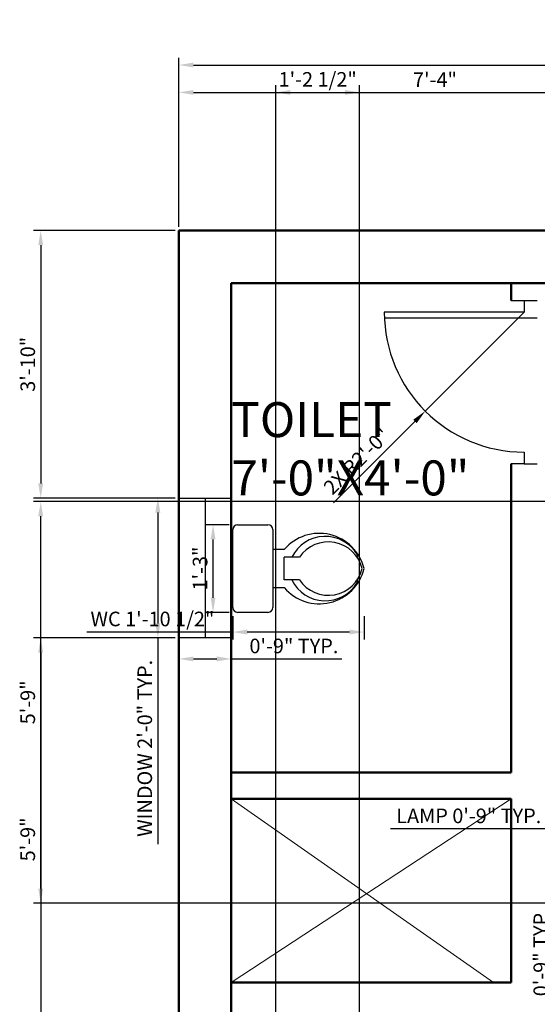
# Model space of a CAD drawing. Units: inches. Extents: x 3242 to 3618, y 1365 to 1814.
# Tile 4 of 6: x 3244 to 3333, y 1626 to 1795. Entities that reach past the tile are written whole.
import ezdxf

# ---------------------------------------------------------------- set-up
doc = ezdxf.new("R2010")
doc.units = ezdxf.units.IN
for name, color, linetype, lineweight in [('A-ANNO-DIMS', 2, 'Continuous', 18), ('A-AREA-IDEN', 7, 'Continuous', 25), ('A-DOOR', 4, 'Continuous', 25), ('A-FLOR-FIXT', 8, 'Continuous', 25), ('A-FLOR-OPEN', 1, 'Continuous', 13), ('A-GLAZ', 5, 'Continuous', 25), ('A-WALL', 7, 'Continuous', 50)]:
    doc.layers.add(name, color=color, linetype=linetype, lineweight=lineweight)
doc.styles.get("Standard").update_dxf_attribs({"font": 'arial.ttf'})
doc.dimstyles.new('ISO-25', dxfattribs={"dimtxt": 2.5, "dimasz": 2.5, "dimexe": 1.25, "dimexo": 0.625, "dimtad": 1, "dimdec": 0, "dimlunit": 3, "dimtxsty": 'Standard', "dimcen": 2.5, "dimadec": 0, "dimazin": 0, "dimtfac": 1, "dimtdec": 0, "dimtmove": 0, "dimatfit": 3, "dimfxl": 1, "dimarcsym": 0})

# ---------------------------------------------------------------- blocks, each defined once
blk = doc.blocks.new('A$C02F3725D')
for p, q in [((0.025, 0.69), (0.435, 0.69)), ((0, 0.505), (0, 0.665)), ((0.46, 0.665), (0.46, 0.505)), ((0.435, 0.48), (0.025, 0.48)), ((0.13, 0.48), (0.13, 0.42)), ((0.33, 0.42), (0.33, 0.48)), ((0.17, 0.34), (0.17, 0.42)), ((0.17, 0.42), (0.29, 0.42)), ((0.29, 0.34), (0.29, 0.42)), ((0.1578, 0.035), (0.1724, 0.035)), ((0.2876, 0.035), (0.3022, 0.035))]:
    blk.add_line(p, q)
for centre, radius, start, end in [((0.025, 0.665), 0.025, 90, 180), ((0.435, 0.665), 0.025, 0, 90), ((0.025, 0.505), 0.025, 180, 270), ((0.435, 0.505), 0.025, 270, 0), ((0.2874, 0.2356), 0.2425, 130.4885, 256.2965), ((0.1726, 0.2356), 0.2425, 283.7035, 49.5115), ((0.2568, 0.2042), 0.196, 116.2742, 239.6668), ((0.2032, 0.2042), 0.196, 300.3332, 63.7258), ((0.2732, 0.1883), 0.1834, 124.2157, 256.394), ((0.1868, 0.1883), 0.1834, 283.606, 55.7843)]:
    blk.add_arc(centre, radius, start, end)
blk = doc.blocks.new('*D3')
at = {"layer": 'A-ANNO-DIMS', "color": 0, "lineweight": -2, "transparency": 16777216}
for p, q in [((3271.48, 1759.28), (3271.48, 1788.3)), ((3592.48, 1759.28), (3592.48, 1788.3)), ((3273.98, 1787.05), (3589.98, 1787.05))]:
    blk.add_line(p, q, dxfattribs=at)
at = {"layer": 'A-ANNO-DIMS', "color": 0, "transparency": 16777216}
for points in [[(3273.98, 1787.47), (3273.98, 1786.64), (3271.48, 1787.05)], [(3589.98, 1787.47), (3589.98, 1786.64), (3592.48, 1787.05)]]:
    blk.add_solid(points, dxfattribs=at)
at = {"layer": 'Defpoints', "color": 0, "transparency": 16777216}
for p in [(3592.48, 1787.05), (3271.48, 1758.66), (3592.48, 1758.66)]:
    blk.add_point(p, dxfattribs=at)
at = {"layer": 'A-ANNO-DIMS', "color": 0, "transparency": 16777216, "insert": (3431.98, 1790.74), "char_height": 6, "attachment_point": 5}
blk.add_mtext('26\'-9"', dxfattribs=at)
blk = doc.blocks.new('DOOR-SWING-24IN')
for p, q in [((21.75, 28), (26.25, 28)), ((24, 28), (24, 26)), ((24, 26), (0, 26)), ((26.25, 25), (0, 25)), ((24, 2), (24, 0)), ((24, 0), (21.75, 0)), ((24, 0), (26.25, 0))]:
    blk.add_line(p, q)
blk.add_arc((24, 26), 24, 180, 270)
blk = doc.blocks.new('WINDOW-24IN')
for p, q in [((0, 9), (24, 9)), ((0, 0), (0, 9)), ((24, 9), (24, 0)), ((0, 4.5), (24, 4.5)), ((24, 0), (0, 0))]:
    blk.add_line(p, q)
blk = doc.blocks.new('*D15')
at = {"layer": 'A-ANNO-DIMS', "color": 0, "lineweight": -2, "transparency": 16777216}
for p, q in [((3270.86, 1712.77), (3266.63, 1712.77)), ((3267.88, 1710.27), (3267.88, 1691.27)), ((3270.86, 1688.77), (3266.63, 1688.77)), ((3267.88, 1688.77), (3267.88, 1653.38))]:
    blk.add_line(p, q, dxfattribs=at)
at = {"layer": 'A-ANNO-DIMS', "color": 0, "transparency": 16777216}
for points in [[(3267.46, 1710.27), (3268.3, 1710.27), (3267.88, 1712.77)], [(3267.46, 1691.27), (3268.3, 1691.27), (3267.88, 1688.77)]]:
    blk.add_solid(points, dxfattribs=at)
at = {"layer": 'Defpoints', "color": 0, "transparency": 16777216}
for p in [(3271.48, 1712.77), (3267.88, 1688.77), (3271.48, 1688.77)]:
    blk.add_point(p, dxfattribs=at)
at = {"layer": 'A-ANNO-DIMS', "color": 0, "transparency": 16777216, "insert": (3265.96, 1669.83), "char_height": 2.5, "attachment_point": 5, "rotation": 90}
blk.add_mtext('WINDOW 2\'-0" TYP.', dxfattribs=at)
blk = doc.blocks.new('*D16')
at = {"layer": 'A-ANNO-DIMS', "color": 0, "lineweight": -2, "transparency": 16777216}
for p, q in [((3271.48, 1688.14), (3271.48, 1683.92)), ((3280.48, 1688.14), (3280.48, 1683.92)), ((3273.98, 1685.17), (3277.98, 1685.17)), ((3280.48, 1685.17), (3299.47, 1685.17))]:
    blk.add_line(p, q, dxfattribs=at)
at = {"layer": 'A-ANNO-DIMS', "color": 0, "transparency": 16777216}
for points in [[(3273.98, 1685.59), (3273.98, 1684.75), (3271.48, 1685.17)], [(3277.98, 1685.59), (3277.98, 1684.75), (3280.48, 1685.17)]]:
    blk.add_solid(points, dxfattribs=at)
at = {"layer": 'Defpoints', "color": 0, "transparency": 16777216}
for p in [(3271.48, 1688.77), (3280.48, 1688.77), (3280.48, 1685.17)]:
    blk.add_point(p, dxfattribs=at)
at = {"layer": 'A-ANNO-DIMS', "color": 0, "transparency": 16777216, "insert": (3291.22, 1687.07), "char_height": 2.5, "attachment_point": 5}
blk.add_mtext('0\'-9" TYP.', dxfattribs=at)
blk = doc.blocks.new('*D21')
at = {"layer": 'A-ANNO-DIMS', "color": 0, "lineweight": -2, "transparency": 16777216}
for p, q in [((3280.73, 1692.53), (3280.73, 1688.53)), ((3303.26, 1692.53), (3303.26, 1688.53)), ((3280.73, 1689.78), (3255.68, 1689.78)), ((3300.76, 1689.78), (3283.23, 1689.78))]:
    blk.add_line(p, q, dxfattribs=at)
at = {"layer": 'A-ANNO-DIMS', "color": 0, "transparency": 16777216}
for points in [[(3283.23, 1690.2), (3283.23, 1689.36), (3280.73, 1689.78)], [(3300.76, 1690.2), (3300.76, 1689.36), (3303.26, 1689.78)]]:
    blk.add_solid(points, dxfattribs=at)
at = {"layer": 'Defpoints', "color": 0, "transparency": 16777216}
for p in [(3280.73, 1693.16), (3303.26, 1693.16), (3280.73, 1689.78)]:
    blk.add_point(p, dxfattribs=at)
at = {"layer": 'A-ANNO-DIMS', "color": 0, "transparency": 16777216, "insert": (3266.95, 1691.7), "char_height": 2.5, "attachment_point": 5}
blk.add_mtext('WC 1\'-10 1/2"', dxfattribs=at)
blk = doc.blocks.new('*D22')
at = {"layer": 'A-ANNO-DIMS', "color": 0, "lineweight": -2, "transparency": 16777216}
for p, q in [((3280.11, 1708.17), (3276.1, 1708.17)), ((3277.35, 1695.66), (3277.35, 1705.67)), ((3280.11, 1693.16), (3276.1, 1693.16))]:
    blk.add_line(p, q, dxfattribs=at)
at = {"layer": 'A-ANNO-DIMS', "color": 0, "transparency": 16777216}
for points in [[(3276.94, 1705.67), (3277.77, 1705.67), (3277.35, 1708.17)], [(3276.94, 1695.66), (3277.77, 1695.66), (3277.35, 1693.16)]]:
    blk.add_solid(points, dxfattribs=at)
at = {"layer": 'Defpoints', "color": 0, "transparency": 16777216}
for p in [(3277.35, 1708.17), (3280.73, 1708.17), (3280.73, 1693.16)]:
    blk.add_point(p, dxfattribs=at)
at = {"layer": 'A-ANNO-DIMS', "color": 0, "transparency": 16777216, "insert": (3275.45, 1700.67), "char_height": 2.5, "attachment_point": 5, "rotation": 90}
blk.add_mtext('1\'-3"', dxfattribs=at)
blk = doc.blocks.new('*D29')
at = {"layer": 'A-ANNO-DIMS', "color": 0, "lineweight": -2, "transparency": 16777216}
for p, q in [((3337.15, 1655.29), (3337.15, 1657.27)), ((3346.15, 1655.29), (3346.15, 1657.27)), ((3337.15, 1656.02), (3307.79, 1656.02)), ((3343.65, 1656.02), (3339.65, 1656.02))]:
    blk.add_line(p, q, dxfattribs=at)
at = {"layer": 'A-ANNO-DIMS', "color": 0, "transparency": 16777216}
for points in [[(3339.65, 1656.43), (3339.65, 1655.6), (3337.15, 1656.02)], [(3343.65, 1656.43), (3343.65, 1655.6), (3346.15, 1656.02)]]:
    blk.add_solid(points, dxfattribs=at)
at = {"layer": 'Defpoints', "color": 0, "transparency": 16777216}
for p in [(3337.15, 1656.02), (3337.15, 1654.67), (3346.15, 1654.67)]:
    blk.add_point(p, dxfattribs=at)
at = {"layer": 'A-ANNO-DIMS', "color": 0, "transparency": 16777216, "insert": (3321.22, 1657.92), "char_height": 2.5, "attachment_point": 5}
blk.add_mtext('LAMP 0\'-9" TYP.', dxfattribs=at)
blk = doc.blocks.new('*D30')
at = {"layer": 'A-ANNO-DIMS', "color": 0, "lineweight": -2, "transparency": 16777216}
for p, q in [((3336.53, 1654.67), (3334.55, 1654.67)), ((3335.8, 1652.17), (3335.8, 1648.17)), ((3336.53, 1645.67), (3334.55, 1645.67)), ((3335.8, 1645.67), (3335.8, 1626.68))]:
    blk.add_line(p, q, dxfattribs=at)
at = {"layer": 'A-ANNO-DIMS', "color": 0, "transparency": 16777216}
for points in [[(3335.39, 1652.17), (3336.22, 1652.17), (3335.8, 1654.67)], [(3335.39, 1648.17), (3336.22, 1648.17), (3335.8, 1645.67)]]:
    blk.add_solid(points, dxfattribs=at)
at = {"layer": 'Defpoints', "color": 0, "transparency": 16777216}
for p in [(3337.15, 1654.67), (3335.8, 1645.67), (3337.15, 1645.67)]:
    blk.add_point(p, dxfattribs=at)
at = {"layer": 'A-ANNO-DIMS', "color": 0, "transparency": 16777216, "insert": (3333.9, 1634.92), "char_height": 2.5, "attachment_point": 5, "rotation": 90}
blk.add_mtext('0\'-9" TYP.', dxfattribs=at)
blk = doc.blocks.new('*D33')
at = {"layer": 'A-ANNO-DIMS', "color": 0, "lineweight": -2, "transparency": 16777216}
for p, q in [((3271.48, 1759.28), (3271.48, 1783.61)), ((3273.98, 1782.36), (3356.86, 1782.36)), ((3359.36, 1759.28), (3359.36, 1783.61))]:
    blk.add_line(p, q, dxfattribs=at)
at = {"layer": 'A-ANNO-DIMS', "color": 0, "transparency": 16777216}
for points in [[(3273.98, 1782.77), (3273.98, 1781.94), (3271.48, 1782.36)], [(3356.86, 1782.77), (3356.86, 1781.94), (3359.36, 1782.36)]]:
    blk.add_solid(points, dxfattribs=at)
at = {"layer": 'Defpoints', "color": 0, "transparency": 16777216}
for p in [(3359.36, 1782.36), (3271.48, 1758.66), (3359.36, 1758.66)]:
    blk.add_point(p, dxfattribs=at)
at = {"layer": 'A-ANNO-DIMS', "color": 0, "transparency": 16777216, "insert": (3315.42, 1784.23), "char_height": 2.5, "attachment_point": 5}
blk.add_mtext('7\'-4"', dxfattribs=at)
blk = doc.blocks.new('*D37')
at = {"layer": 'A-ANNO-DIMS', "color": 0, "lineweight": -2, "transparency": 16777216}
for p, q in [((3270.86, 1758.66), (3246.53, 1758.66)), ((3247.78, 1756.16), (3247.78, 1715.27)), ((3270.86, 1712.77), (3246.53, 1712.77))]:
    blk.add_line(p, q, dxfattribs=at)
at = {"layer": 'A-ANNO-DIMS', "color": 0, "transparency": 16777216}
for points in [[(3247.36, 1756.16), (3248.2, 1756.16), (3247.78, 1758.66)], [(3247.36, 1715.27), (3248.2, 1715.27), (3247.78, 1712.77)]]:
    blk.add_solid(points, dxfattribs=at)
at = {"layer": 'Defpoints', "color": 0, "transparency": 16777216}
for p in [(3271.48, 1758.66), (3247.78, 1712.77), (3271.48, 1712.77)]:
    blk.add_point(p, dxfattribs=at)
at = {"layer": 'A-ANNO-DIMS', "color": 0, "transparency": 16777216, "insert": (3245.88, 1735.71), "char_height": 2.5, "attachment_point": 5, "rotation": 90}
blk.add_mtext('3\'-10"', dxfattribs=at)
blk = doc.blocks.new('*D38')
at = {"layer": 'A-ANNO-DIMS', "color": 0, "lineweight": -2, "transparency": 16777216}
for p, q in [((3270.86, 1688.77), (3246.53, 1688.77)), ((3247.78, 1686.27), (3247.78, 1622.15)), ((3270.86, 1619.65), (3246.53, 1619.65))]:
    blk.add_line(p, q, dxfattribs=at)
at = {"layer": 'A-ANNO-DIMS', "color": 0, "transparency": 16777216}
for points in [[(3247.36, 1686.27), (3248.2, 1686.27), (3247.78, 1688.77)], [(3247.36, 1622.15), (3248.2, 1622.15), (3247.78, 1619.65)]]:
    blk.add_solid(points, dxfattribs=at)
at = {"layer": 'Defpoints', "color": 0, "transparency": 16777216}
for p in [(3271.48, 1688.77), (3247.78, 1619.65), (3271.48, 1619.65)]:
    blk.add_point(p, dxfattribs=at)
at = {"layer": 'A-ANNO-DIMS', "color": 0, "transparency": 16777216, "insert": (3245.88, 1654.21), "char_height": 2.5, "attachment_point": 5, "rotation": 90}
blk.add_mtext('5\'-9"', dxfattribs=at)
blk = doc.blocks.new('*D52')
at = {"layer": 'A-ANNO-DIMS', "color": 0, "lineweight": -2, "transparency": 16777216}
for p, q in [((3335.29, 1712.15), (3246.53, 1712.15)), ((3247.78, 1645.78), (3247.78, 1709.65)), ((3335.29, 1643.28), (3246.53, 1643.28))]:
    blk.add_line(p, q, dxfattribs=at)
at = {"layer": 'A-ANNO-DIMS', "color": 0, "transparency": 16777216}
for points in [[(3247.36, 1709.65), (3248.2, 1709.65), (3247.78, 1712.15)], [(3247.36, 1645.78), (3248.2, 1645.78), (3247.78, 1643.28)]]:
    blk.add_solid(points, dxfattribs=at)
at = {"layer": 'Defpoints', "color": 0, "transparency": 16777216}
for p in [(3247.78, 1712.15), (3335.91, 1712.15), (3335.91, 1643.28)]:
    blk.add_point(p, dxfattribs=at)
at = {"layer": 'A-ANNO-DIMS', "color": 0, "transparency": 16777216, "insert": (3245.88, 1677.72), "char_height": 2.5, "attachment_point": 5, "rotation": 90}
blk.add_mtext('5\'-9"', dxfattribs=at)
blk = doc.blocks.new('*D56')
at = {"layer": 'A-ANNO-DIMS', "color": 0, "lineweight": -2, "transparency": 16777216}
for p, q in [((3288.1, 1513.62), (3288.1, 1783.61)), ((3290.6, 1782.36), (3300, 1782.36)), ((3302.5, 1513.62), (3302.5, 1783.61))]:
    blk.add_line(p, q, dxfattribs=at)
at = {"layer": 'A-ANNO-DIMS', "color": 0, "transparency": 16777216}
for points in [[(3290.6, 1782.77), (3290.6, 1781.94), (3288.1, 1782.36)], [(3300, 1782.77), (3300, 1781.94), (3302.5, 1782.36)]]:
    blk.add_solid(points, dxfattribs=at)
at = {"layer": 'Defpoints', "color": 0, "transparency": 16777216}
for p in [(3302.5, 1782.36), (3288.1, 1513), (3302.5, 1513)]:
    blk.add_point(p, dxfattribs=at)
at = {"layer": 'A-ANNO-DIMS', "color": 0, "transparency": 16777216, "insert": (3295.3, 1784.27), "char_height": 2.5, "attachment_point": 5}
blk.add_mtext('1\'-2 1/2"', dxfattribs=at)
blk = doc.blocks.new('*D66')
at = {"layer": 'A-ANNO-DIMS', "color": 0, "lineweight": -2, "transparency": 16777216}
for p, q in [((3330.73, 1744.66), (3313.76, 1727.68)), ((3298.03, 1711.95), (3311.99, 1725.92))]:
    blk.add_line(p, q, dxfattribs=at)
at = {"layer": 'A-ANNO-DIMS', "color": 0, "transparency": 16777216}
blk.add_solid([(3311.7, 1726.21), (3312.29, 1725.62), (3313.76, 1727.68)], dxfattribs=at)
at = {"layer": 'Defpoints', "color": 0, "transparency": 16777216}
for p in [(3330.73, 1744.66), (3313.76, 1727.68)]:
    blk.add_point(p, dxfattribs=at)
at = {"layer": 'A-ANNO-DIMS', "color": 0, "transparency": 16777216, "insert": (3302.23, 1718.85), "char_height": 2.5, "attachment_point": 5, "rotation": 45.0005}
blk.add_mtext('2X R2\'-0"', dxfattribs=at)

msp = doc.modelspace()

# ---------------------------------------------------------------- linework, layer by layer
at = {"layer": 'A-FLOR-OPEN'}
for p, q in [((3280.48, 1661.16), (3325.48, 1629.66)), ((3328.48, 1661.16), (3280.48, 1629.66))]:
    msp.add_line(p, q, dxfattribs=at)
at = {"layer": 'A-WALL'}
for p, q in [((3271.48, 1758.66), (3271.48, 1401.66)), ((3271.48, 1758.66), (3592.48, 1758.66)), ((3280.48, 1749.66), (3583.48, 1749.66)), ((3280.48, 1749.66), (3280.48, 1410.66)), ((3328.48, 1749.66), (3328.48, 1746.66)), ((3328.48, 1718.66), (3328.48, 1665.66)), ((3280.48, 1665.66), (3328.48, 1665.66)), ((3280.48, 1661.16), (3328.48, 1661.16)), ((3328.48, 1661.16), (3328.48, 1629.66)), ((3280.48, 1629.66), (3297.48, 1629.66)), ((3297.48, 1629.66), (3325.48, 1629.66)), ((3325.48, 1629.66), (3328.48, 1629.66))]:
    msp.add_line(p, q, dxfattribs=at)

# ---------------------------------------------------------------- block references
at = {"layer": 'A-DOOR'}
msp.add_blockref('DOOR-SWING-24IN', (3306.73, 1718.65), dxfattribs=at)
at = {"layer": 'A-FLOR-FIXT', "xscale": 32.64316118045935, "yscale": 32.64316118045935, "zscale": 32.64316118045935, "rotation": 90}
msp.add_blockref('A$C02F3725D', (3303.26, 1693.16), dxfattribs=at)
at = {"layer": 'A-GLAZ', "rotation": 270.0000000000025}
msp.add_blockref('WINDOW-24IN', (3271.48, 1712.77), dxfattribs=at)

# ---------------------------------------------------------------- texts
at = {"layer": 'A-AREA-IDEN', "insert": (3280.48, 1729.22), "char_height": 6, "attachment_point": 1}
msp.add_mtext('TOILET\\P7\'-0"X4\'-0"', dxfattribs=at)

# ---------------------------------------------------------------- dimensions: what is measured, and where the dimension line sits
at = {"layer": 'A-ANNO-DIMS'}
for base, p1, p2, override, picture, middle in [((3592.48, 1787.05), (3271.48, 1758.66), (3592.48, 1758.66), {"dimtxt": 6, "dimclrd": 0, "dimclre": 0, "dimclrt": 0}, '*D3', (3431.98, 1790.74)), ((3302.5, 1782.36), (3288.1, 1513), (3302.5, 1513), {"dimdec": 1, "dimlfac": 1, "dimrnd": 0, "dimzin": 1, "dimdsep": 46, "dimlunit": 4, "dimfrac": 2}, '*D56', (3295.3, 1784.27)), ((3359.36, 1782.36), (3271.48, 1758.66), (3359.36, 1758.66), {"dimdec": 1, "dimlfac": 1, "dimrnd": 0, "dimzin": 1, "dimdsep": 46, "dimlunit": 4, "dimfrac": 2}, '*D33', (3315.42, 1784.23))]:
    dim = msp.add_linear_dim(base=base, p1=p1, p2=p2, dimstyle='ISO-25', override=override, dxfattribs=at)
    dim.commit()
    dim.dimension.update_dxf_attribs({"geometry": picture, "text_midpoint": middle})
for base, p1, p2, picture, middle in [((3247.78, 1712.77), (3271.48, 1758.66), (3271.48, 1712.77), '*D37', (3245.88, 1735.71)), ((3247.78, 1712.15), (3335.91, 1643.28), (3335.91, 1712.15), '*D52', (3245.88, 1677.72)), ((3277.35, 1708.17), (3280.73, 1693.16), (3280.73, 1708.17), '*D22', (3275.45, 1700.67)), ((3247.78, 1619.65), (3271.48, 1688.77), (3271.48, 1619.65), '*D38', (3245.88, 1654.21))]:
    dim = msp.add_linear_dim(base=base, p1=p1, p2=p2, angle=90, dimstyle='ISO-25', override={"dimdec": 1, "dimlfac": 1, "dimrnd": 0, "dimzin": 1, "dimdsep": 46, "dimlunit": 4, "dimfrac": 2}, dxfattribs=at)
    dim.commit()
    dim.dimension.update_dxf_attribs({"geometry": picture, "text_midpoint": middle})
dim = msp.add_radius_dim(center=(3330.73, 1744.66), mpoint=(3313.76, 1727.68), text='2X <>', dimstyle='ISO-25', override={"dimdec": 1, "dimlfac": 1, "dimrnd": 0, "dimzin": 1, "dimdsep": 46, "dimlunit": 4, "dimfrac": 2}, dxfattribs=at)
dim.commit()
dim.dimension.update_dxf_attribs({"geometry": '*D66', "text_midpoint": (3303.58, 1717.5), "dimtype": 164})
for base, p1, p2, angle, text, picture, middle in [((3267.88, 1688.77), (3271.48, 1712.77), (3271.48, 1688.77), 270, 'WINDOW <> TYP.', '*D15', (3265.96, 1669.83)), ((3280.73, 1689.78), (3303.26, 1693.16), (3280.73, 1693.16), 180, 'WC <>', '*D21', (3266.95, 1691.7)), ((3280.48, 1685.17), (3271.48, 1688.77), (3280.48, 1688.77), 0, '<> TYP.', '*D16', (3291.22, 1687.07)), ((3337.15, 1656.02), (3346.15, 1654.67), (3337.15, 1654.67), 180, 'LAMP <> TYP.', '*D29', (3321.22, 1657.92)), ((3335.8, 1645.67), (3337.15, 1654.67), (3337.15, 1645.67), 270, '<> TYP.', '*D30', (3333.9, 1634.92))]:
    dim = msp.add_linear_dim(base=base, p1=p1, p2=p2, angle=angle, text=text, dimstyle='ISO-25', override={"dimdec": 1, "dimlfac": 1, "dimrnd": 0, "dimzin": 1, "dimdsep": 46, "dimlunit": 4, "dimfrac": 2}, dxfattribs=at)
    dim.commit()
    dim.dimension.update_dxf_attribs({"geometry": picture, "text_midpoint": middle})

doc.saveas('drawing.dxf')
